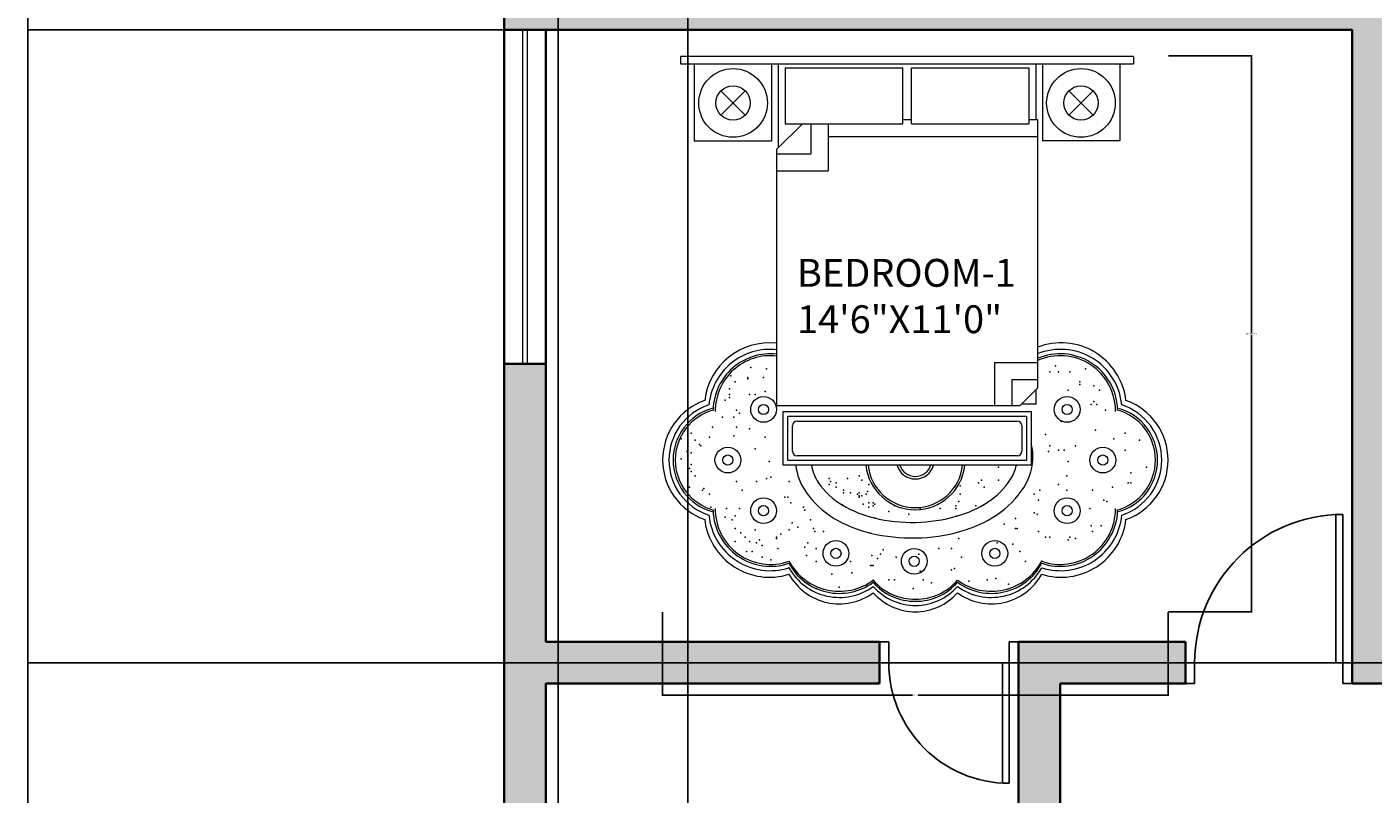
# Model space of a CAD drawing. Units: inches. Extents: x 5716 to 6907, y 12769 to 13594.
# Tile 6 of 17: x 5716 to 6007, y 13266 to 13432. Entities that reach past the tile are written whole.
import ezdxf

# ---------------------------------------------------------------- set-up
doc = ezdxf.new("R2010")
doc.units = ezdxf.units.IN
for name, color, linetype, lineweight in [('A-ANNO-DIMS', 2, 'Continuous', 18), ('A-AREA-IDEN', 7, 'Continuous', 18), ('A-DOOR', 4, 'Continuous', 25), ('A-FURN', 8, 'Continuous', 18), ('A-GLAZ', 4, 'Continuous', 18), ('A-WALL', 7, 'Continuous', 35), ('A-WALL-PATT', 252, 'Continuous', 13)]:
    doc.layers.add(name, color=color, linetype=linetype, lineweight=lineweight)
doc.styles.get("Standard").update_dxf_attribs({"font": 'arial.ttf'})
doc.dimstyles.get("Standard").update_dxf_attribs({"dimtxt": 0.18, "dimasz": 0.18, "dimexe": 0.18, "dimexo": 0.0625, "dimgap": 0.09, "dimtad": 0, "dimtih": 1, "dimtoh": 1, "dimdec": 4, "dimzin": 0, "dimdsep": 46, "dimtxsty": 'Standard', "dimcen": 0.09, "dimadec": 0, "dimazin": 0, "dimtfac": 1, "dimtdec": 4, "dimtofl": 0, "dimtmove": 0, "dimatfit": 3, "dimfxl": 1, "dimtolj": 1, "dimtzin": 0, "dimarcsym": 0})

# ---------------------------------------------------------------- blocks, each defined once
blk = doc.blocks.new('A$C1EC128A1')
for p, q in [((0.1147, 3.56), (3.0187, 3.56)), ((0.1147, 3.555), (0.1147, 3.511)), ((3.0187, 3.555), (3.0187, 3.511)), ((0.1147, 3.511), (3.0187, 3.511)), ((0.2027, 3.511), (0.2027, 3.4616)), ((0.2027, 3.4601), (0.2027, 3.016)), ((0.6977, 3.511), (0.6977, 3.016)), ((0.7417, 3.511), (0.7417, 2.972)), ((0.7857, 3.4835), (1.5392, 3.4835)), ((0.7857, 3.4835), (0.7857, 3.126)), ((1.5392, 3.126), (1.5392, 3.4835)), ((1.5942, 3.126), (1.5942, 3.4835)), ((1.5942, 3.4835), (2.3477, 3.4835)), ((2.3477, 3.4835), (2.3477, 3.126)), ((2.3917, 3.511), (2.3917, 3.1535)), ((2.4357, 3.511), (2.4357, 3.016)), ((2.9307, 3.511), (2.9307, 3.016)), ((0.3741, 3.1815), (0.5297, 3.337)), ((0.3741, 3.337), (0.5297, 3.1815)), ((2.6038, 3.337), (2.7594, 3.1815)), ((2.7594, 3.337), (2.6038, 3.1815)), ((0.7307, 2.961), (0.8957, 3.126)), ((0.7857, 3.126), (1.5392, 3.126)), ((0.9507, 3.126), (0.9507, 2.9335)), ((1.0607, 3.126), (1.0607, 2.8235)), ((1.5392, 3.1535), (1.5942, 3.1535)), ((1.5942, 3.126), (2.3477, 3.126)), ((2.3477, 3.1535), (2.4027, 3.1535)), ((2.4027, 3.1535), (2.4027, 1.432)), ((1.0607, 3.0435), (2.4027, 3.0435)), ((0.2027, 3.016), (0.6977, 3.016)), ((0.7307, 2.961), (0.7307, 1.322)), ((2.9307, 3.016), (2.4357, 3.016)), ((0.7307, 2.9335), (0.9507, 2.9335)), ((0.7307, 2.8235), (1.0607, 2.8235)), ((2.1277, 1.597), (2.4027, 1.597)), ((2.1277, 1.597), (2.1277, 1.322)), ((2.2377, 1.487), (2.2377, 1.322)), ((2.2377, 1.487), (2.4027, 1.487)), ((2.2927, 1.322), (2.4027, 1.432)), ((2.3917, 1.421), (2.3917, 1.333)), ((0.7307, 1.322), (2.2927, 1.322)), ((2.3037, 1.333), (2.3917, 1.333)), ((0.7721, 1.282), (2.3633, 1.282)), ((0.7721, 0.939), (0.7721, 1.282)), ((0.8021, 1.252), (2.3333, 1.252)), ((0.8021, 0.969), (0.8021, 1.252)), ((0.8621, 1.222), (2.2733, 1.222)), ((2.3333, 1.252), (2.3333, 0.969)), ((2.3633, 1.282), (2.3633, 0.939)), ((0.8321, 1.029), (0.8321, 1.192)), ((2.3033, 1.192), (2.3033, 1.029)), ((2.3333, 0.969), (0.8021, 0.969)), ((2.2733, 0.999), (0.8621, 0.999)), ((2.3633, 0.939), (0.7721, 0.939))]:
    blk.add_line(p, q)
for centre, radius in [((0.4519, 3.2593), 0.22), ((2.6816, 3.2593), 0.22), ((0.4519, 3.2593), 0.11), ((2.6816, 3.2593), 0.11), ((0.647, 1.2961), 0.0826), ((0.647, 1.2961), 0.0326), ((2.593, 1.2961), 0.0826), ((2.593, 1.2961), 0.0326), ((0.4183, 0.9718), 0.0826), ((2.8217, 0.9718), 0.0826), ((0.4183, 0.9718), 0.0326), ((2.8217, 0.9718), 0.0326), ((0.647, 0.6475), 0.0826), ((2.593, 0.6475), 0.0826), ((0.647, 0.6475), 0.0326), ((2.593, 0.6475), 0.0326), ((1.1109, 0.3741), 0.0826), ((2.1291, 0.3741), 0.0826), ((1.1109, 0.3741), 0.0326), ((1.6128, 0.3232), 0.0826), ((1.6128, 0.3232), 0.0326), ((2.1291, 0.3741), 0.0326)]:
    blk.add_circle(centre, radius)
for centre, radius, start, end in [((0.6854, 1.3045), 0.4183, 83.78243, 173.25148), ((0.6884, 1.2877), 0.3932, 83.81567, 174.52996), ((0.6921, 1.2838), 0.369, 83.99709, 177.99757), ((0.6913, 1.2866), 0.3539, 83.60511, 180.66989), ((2.5546, 1.3045), 0.4183, 6.74852, 111.27952), ((2.5516, 1.2877), 0.3932, 5.47004, 112.24899), ((2.5479, 1.2838), 0.369, 2.00243, 113.15364), ((2.5487, 1.2866), 0.3539, 359.33011, 114.35507), ((0.4048, 0.972), 0.4048, 109.45268, 180), ((0.4119, 0.972), 0.3714, 108.02557, 180), ((0.411, 0.972), 0.3435, 105.78906, 180), ((2.829, 0.972), 0.3435, 0, 74.21094), ((2.8281, 0.972), 0.3714, 0, 71.97443), ((2.8352, 0.972), 0.4048, 0, 70.54732), ((0.4122, 0.972), 0.3312, 104.76604, 180), ((0.8621, 1.192), 0.03, 90, 180), ((2.2733, 1.192), 0.03, 0, 90), ((2.8278, 0.972), 0.3312, 0, 75.23396), ((2.0084, 0.9935), 0.365, 1.17824, 13.48124), ((0.4048, 0.972), 0.4048, 180, 250.54732), ((0.4119, 0.972), 0.3714, 180, 251.97443), ((0.411, 0.972), 0.3435, 180, 254.21094), ((0.4122, 0.972), 0.3312, 180, 255.23396), ((0.8621, 1.029), 0.03, 180, 270), ((2.2733, 1.029), 0.03, 270, 0), ((2.0084, 0.9935), 0.365, 327.62391, 1.17824), ((2.8278, 0.972), 0.3312, 284.76604, 0), ((2.829, 0.972), 0.3435, 285.78906, 0), ((2.8281, 0.972), 0.3714, 288.02557, 0), ((2.8352, 0.972), 0.4048, 289.45268, 0), ((1.2169, 0.9773), 0.365, 186.01972, 214.73257), ((1.2169, 0.9773), 0.265, 188.30546, 214.73257), ((1.62, 0.972), 0.3185, 185.95071, 354.04929), ((1.62, 0.972), 0.305, 186.21512, 353.78488), ((1.62, 0.972), 0.1215, 195.7695, 344.2305), ((1.62, 0.972), 0.105, 198.32909, 341.67091), ((2.0084, 0.9935), 0.265, 327.62391, 348.11864), ((1.4035, 1.1066), 0.492, 214.73257, 239.1926), ((1.8167, 1.1151), 0.492, 303.16388, 327.62391), ((1.8167, 1.1151), 0.592, 303.16388, 327.62391), ((1.4035, 1.1066), 0.592, 214.73257, 239.1926), ((1.6878, 1.3123), 0.7275, 285.68186, 303.16388), ((0.6884, 0.6563), 0.3932, 185.47004, 288.01752), ((0.6921, 0.6602), 0.369, 182.00243, 288.62304), ((0.6913, 0.6574), 0.3539, 179.33011, 289.59453), ((1.5241, 1.3089), 0.7275, 239.1926, 256.67462), ((1.5995, 1.627), 1.0544, 271.17824, 285.68186), ((1.6878, 1.3123), 0.8275, 285.68186, 303.16388), ((2.5487, 0.6574), 0.3539, 250.40547, 0.66989), ((2.5479, 0.6602), 0.369, 251.37696, 357.99757), ((2.5516, 0.6563), 0.3932, 251.98248, 354.52996), ((0.6854, 0.6395), 0.4183, 186.74852, 287.32326), ((1.5241, 1.3089), 0.8275, 239.1926, 256.67462), ((1.5995, 1.627), 1.0544, 256.67462, 271.17824), ((2.5546, 0.6395), 0.4183, 252.67674, 353.25148), ((1.5995, 1.627), 1.1544, 256.67462, 271.17824), ((1.5995, 1.627), 1.1544, 271.17824, 285.68186), ((1.1328, 0.4977), 0.3665, 208.29135, 306.34788), ((1.1328, 0.4842), 0.3665, 208.29135, 306.34788), ((1.133, 0.4609), 0.369, 208.93019, 306.02618), ((2.1072, 0.4977), 0.3665, 233.65212, 331.70865), ((2.1072, 0.4842), 0.3665, 233.65212, 331.70865), ((2.107, 0.4609), 0.369, 233.97382, 331.06981), ((1.1324, 0.4204), 0.3694, 209.22014, 306.07902), ((1.6145, 0.4295), 0.3486, 220.6393, 270.90521), ((1.6145, 0.416), 0.3486, 220.6393, 270.90521), ((1.6255, 0.4295), 0.3486, 269.09479, 319.3607), ((1.6255, 0.416), 0.3486, 269.09479, 319.3607), ((2.1076, 0.4204), 0.3694, 233.92098, 330.77986), ((1.62, 0.4004), 0.3599, 221.38778, 270), ((1.62, 0.36), 0.36, 221.41854, 270), ((1.62, 0.4004), 0.3599, 270, 318.61222), ((1.62, 0.36), 0.36, 270, 318.58146)]:
    blk.add_arc(centre, radius, start, end)
for p in [(0.5654, 1.5652), (0.6657, 1.5561), (2.5184, 1.5744), (2.71, 1.5561), (0.4376, 1.5104), (0.465, 1.4739), (0.5471, 1.5013), (0.5471, 1.4922), (0.6475, 1.5013), (2.4819, 1.5378), (2.5366, 1.5378), (2.6097, 1.5378), (2.6735, 1.4739), (0.4285, 1.4282), (0.4285, 1.3917), (0.5562, 1.3917), (0.5927, 1.3917), (0.6566, 1.41), (2.6005, 1.4191), (2.6735, 1.4556), (2.7648, 1.4465), (2.8013, 1.4191), (0.4011, 1.3552), (0.4285, 1.3734), (2.3917, 1.333), (2.7465, 1.3278), (2.7648, 1.346), (2.7831, 1.3278), (0.3828, 1.2456), (0.4558, 1.2456), (0.4741, 1.2912), (0.4923, 1.273), (2.5549, 1.2182), (2.8378, 1.2912), (0.1821, 1.1451), (0.3189, 1.1816), (0.4558, 1.1268), (0.4741, 1.1816), (0.5562, 1.1725), (2.4545, 1.1359), (2.7739, 1.1634), (2.9656, 1.1451), (0.1182, 1.1085), (0.2094, 1.0994), (0.2368, 1.072), (0.2459, 1.0629), (0.3007, 1.1177), (0.5927, 1.0446), (0.6566, 1.1177), (2.4819, 1.0629), (2.5366, 1.0355), (2.5731, 1.0355), (2.6462, 1.0629), (2.8926, 1.1085), (2.9656, 1.0355), (3.0568, 1.0994), (0.1182, 0.9807), (0.1547, 1.0263), (0.1821, 1.0172), (0.684, 0.9624), (2.4728, 1.0263), (2.6005, 0.9624), (0.1729, 0.9167), (0.1821, 0.9441), (0.1821, 0.8985), (0.2094, 0.8711), (1.259, 0.8711), (1.3032, 0.939), (1.3168, 0.939), (2.1533, 0.9259), (2.5914, 0.8711), (3.0021, 0.8893), (3.1025, 0.9259), (0.1729, 0.798), (0.2551, 0.7797), (0.2642, 0.7889), (0.4741, 0.8345), (0.5106, 0.7797), (0.6019, 0.8345), (0.6657, 0.8528), (0.6931, 0.8619), (0.8118, 0.8345), (0.9992, 0.8263), (1.0673, 0.8528), (1.0673, 0.8163), (1.0764, 0.8345), (1.1129, 0.8254), (1.1129, 0.798), (1.1586, 0.7797), (1.1859, 0.8528), (1.2772, 0.8437), (1.3228, 0.8163), (1.9069, 0.8071), (2.0256, 0.8254), (2.0438, 0.8437), (2.0438, 0.8437), (2.0621, 0.798), (2.1533, 0.8437), (2.418, 0.7797), (2.5366, 0.8163), (2.5914, 0.7797), (2.7557, 0.7797), (2.8834, 0.798), (2.9838, 0.8254), (3.0021, 0.8254), (0.3007, 0.7523), (0.7844, 0.7341), (0.8026, 0.7341), (0.8209, 0.6975), (1.1586, 0.7615), (1.2042, 0.7615), (1.2498, 0.7523), (1.259, 0.7615), (1.259, 0.7432), (1.259, 0.7341), (1.2772, 0.7432), (1.3046, 0.7523), (1.3137, 0.7706), (1.3228, 0.6975), (1.3502, 0.6975), (1.8978, 0.7067), (1.9069, 0.7523), (2.0858, 0.7033), (2.3815, 0.7523), (2.4089, 0.7158), (2.8287, 0.7158), (2.8469, 0.7067), (0.3098, 0.6701), (0.4011, 0.6062), (0.4102, 0.661), (0.465, 0.6153), (0.4923, 0.661), (0.903, 0.6701), (0.9122, 0.6519), (1.1515, 0.684), (1.1515, 0.684), (1.1515, 0.684), (1.2863, 0.6884), (1.3228, 0.6701), (1.3502, 0.6793), (1.3593, 0.6884), (1.4506, 0.6427), (1.4871, 0.6793), (1.5784, 0.6245), (1.6514, 0.661), (1.6514, 0.661), (1.7792, 0.661), (1.8795, 0.6793), (1.8795, 0.661), (1.8845, 0.6118), (2.0073, 0.6793), (2.3815, 0.6336), (2.3997, 0.6245), (2.7374, 0.661), (0.4467, 0.5879), (0.465, 0.5331), (0.5927, 0.524), (0.8118, 0.524), (0.83, 0.5696), (0.8665, 0.5422), (0.9487, 0.5879), (0.9669, 0.5331), (1.3564, 0.601), (2.1898, 0.5605), (2.2629, 0.597), (2.2629, 0.5331), (2.272, 0.5331), (2.7465, 0.5514), (2.8104, 0.5514), (0.465, 0.4509), (0.5015, 0.5057), (0.5289, 0.4783), (0.5562, 0.4509), (0.6019, 0.4418), (0.6201, 0.46), (0.7296, 0.4783), (0.7296, 0.4692), (0.757, 0.4966), (0.9304, 0.4418), (0.976, 0.5148), (1.0308, 0.5148), (1.3334, 0.5037), (1.8978, 0.4692), (2.1442, 0.4418), (2.2446, 0.4326), (2.4089, 0.5148), (2.4545, 0.4783), (2.4819, 0.4783), (2.6005, 0.46), (2.6097, 0.4783), (2.6462, 0.4692), (2.7557, 0.5148), (0.538, 0.387), (0.5745, 0.387), (0.6384, 0.4235), (0.6384, 0.3504), (0.7388, 0.4052), (0.7388, 0.4052), (0.9122, 0.4144), (0.9213, 0.3596), (0.9852, 0.4052), (1.3411, 0.3596), (1.3959, 0.3687), (1.4141, 0.3961), (1.4962, 0.3504), (1.6423, 0.3687), (1.77, 0.4052), (1.8522, 0.4052), (1.9161, 0.3504), (2.2902, 0.387), (0.6931, 0.3322), (0.81, 0.2824), (0.9852, 0.323), (1.2042, 0.323), (1.332, 0.2956), (1.3411, 0.2956), (1.3502, 0.2956), (1.3776, 0.3413), (1.6514, 0.2591), (1.8522, 0.2682), (1.8704, 0.2774), (2.3267, 0.323), (2.43, 0.324), (1.0856, 0.2408), (1.2133, 0.25), (1.35, 0.2025), (1.4506, 0.2043), (1.4871, 0.2043), (1.6696, 0.2043), (1.7244, 0.186), (1.9617, 0.1952), (2.0803, 0.2043), (2.1351, 0.2134), (2.2172, 0.1769), (0.9852, 0.1495), (1.1312, 0.1586), (1.6058, 0.1495)]:
    blk.add_point(p)
blk = doc.blocks.new('DOOR-SWING-30IN')
for p, q in [((0, 4.5), (-2, 4.5)), ((0, 0), (0, 4.5)), ((26, 0), (26, 4.5)), ((26, 4.5), (28, 4.5)), ((-2, 0), (0, 0)), ((0, -26), (0, 0)), ((0, 0), (1.5, 0)), ((1.5, -25.96), (1.5, 0)), ((28, 0), (26, 0))]:
    blk.add_line(p, q)
blk.add_arc((0, 0), 26, 270, 0)
blk = doc.blocks.new('DOOR-SWING-36IN')
for p, q in [((0, 32), (0, 0)), ((1.5, 31.96), (1.5, 0)), ((-2, 0), (0, 0)), ((0, 0), (0, -4.5)), ((0, 0), (1.5, 0)), ((34, 0), (32, 0)), ((32, 0), (32, -4.5)), ((0, -4.5), (-2, -4.5)), ((32, -4.5), (34, -4.5))]:
    blk.add_line(p, q)
blk.add_arc((0, 0), 32, 0, 90)
blk = doc.blocks.new('WIN-GLAZING-72IN')
for p, q in [((0, 0), (0, -72)), ((1, 0), (1, -72))]:
    blk.add_line(p, q)
blk = doc.blocks.new('*D27')
at = {"layer": 'A-ANNO-DIMS', "color": 0, "lineweight": -2, "transparency": 16777216}
for p, q in [((5962.35, 13425.52), (5980.45, 13425.52)), ((5980.27, 13425.34), (5980.27, 13365.77)), ((5980.27, 13305.83), (5980.27, 13365.4)), ((5962.35, 13305.65), (5980.45, 13305.65))]:
    blk.add_line(p, q, dxfattribs=at)
at = {"layer": 'A-ANNO-DIMS', "color": 0, "transparency": 16777216}
for points in [[(5980.24, 13425.34), (5980.3, 13425.34), (5980.27, 13425.52)], [(5980.24, 13305.83), (5980.3, 13305.83), (5980.27, 13305.65)]]:
    blk.add_solid(points, dxfattribs=at)
at = {"layer": 'Defpoints', "color": 0, "transparency": 16777216}
for p in [(5962.29, 13425.52), (5980.27, 13425.52), (5962.29, 13305.65)]:
    blk.add_point(p, dxfattribs=at)
at = {"layer": 'A-ANNO-DIMS', "color": 0, "transparency": 16777216, "insert": (5980.27, 13365.59), "char_height": 0.18, "attachment_point": 5}
blk.add_mtext('\\A1;BED GROUP 120 TYP.', dxfattribs=at)
blk = doc.blocks.new('*D28')
at = {"layer": 'A-ANNO-DIMS', "color": 0, "lineweight": -2, "transparency": 16777216}
for p, q in [((5853.2, 13305.59), (5853.2, 13287.49)), ((5962.29, 13305.59), (5962.29, 13287.49)), ((5853.38, 13287.67), (5907.16, 13287.67)), ((5962.11, 13287.67), (5908.34, 13287.67))]:
    blk.add_line(p, q, dxfattribs=at)
at = {"layer": 'A-ANNO-DIMS', "color": 0, "transparency": 16777216}
for points in [[(5853.38, 13287.7), (5853.38, 13287.64), (5853.2, 13287.67)], [(5962.11, 13287.7), (5962.11, 13287.64), (5962.29, 13287.67)]]:
    blk.add_solid(points, dxfattribs=at)
at = {"layer": 'Defpoints', "color": 0, "transparency": 16777216}
for p in [(5853.2, 13305.65), (5962.29, 13305.65), (5962.29, 13287.67)]:
    blk.add_point(p, dxfattribs=at)
at = {"layer": 'A-ANNO-DIMS', "color": 0, "transparency": 16777216, "insert": (5907.75, 13287.67), "char_height": 0.18, "attachment_point": 5}
blk.add_mtext('\\A1;109 TYP.', dxfattribs=at)
blk = doc.blocks.new('*D50')
at = {"layer": 'A-ANNO-DIMS', "color": 0, "lineweight": -2, "transparency": 16777216}
for p, q in [((5818.96, 13440.15), (5716.04, 13440.15)), ((5716.22, 13439.97), (5716.22, 13140.83)), ((5716.22, 12841.33), (5716.22, 13140.47)), ((5818.96, 12841.15), (5716.04, 12841.15))]:
    blk.add_line(p, q, dxfattribs=at)
at = {"layer": 'A-ANNO-DIMS', "color": 0, "transparency": 16777216}
for points in [[(5716.19, 13439.97), (5716.25, 13439.97), (5716.22, 13440.15)], [(5716.19, 12841.33), (5716.25, 12841.33), (5716.22, 12841.15)]]:
    blk.add_solid(points, dxfattribs=at)
at = {"layer": 'Defpoints', "color": 0, "transparency": 16777216}
for p in [(5716.22, 13440.15), (5819.02, 13440.15), (5819.02, 12841.15)]:
    blk.add_point(p, dxfattribs=at)
at = {"layer": 'A-ANNO-DIMS', "color": 0, "transparency": 16777216, "insert": (5716.22, 13140.65), "char_height": 0.18, "attachment_point": 5}
blk.add_mtext('\\A1;599', dxfattribs=at)
blk = doc.blocks.new('*D51')
at = {"layer": 'A-ANNO-DIMS', "color": 0, "lineweight": -2, "transparency": 16777216}
for p, q in [((5819.02, 13440.21), (5819.02, 13594.38)), ((5819.2, 13594.2), (6033.23, 13594.2)), ((6247.84, 13594.2), (6033.82, 13594.2)), ((6248.02, 13194.21), (6248.02, 13594.38))]:
    blk.add_line(p, q, dxfattribs=at)
at = {"layer": 'A-ANNO-DIMS', "color": 0, "transparency": 16777216}
for points in [[(5819.2, 13594.23), (5819.2, 13594.17), (5819.02, 13594.2)], [(6247.84, 13594.23), (6247.84, 13594.17), (6248.02, 13594.2)]]:
    blk.add_solid(points, dxfattribs=at)
at = {"layer": 'Defpoints', "color": 0, "transparency": 16777216}
for p in [(6248.02, 13594.2), (5819.02, 13440.15), (6248.02, 13194.15)]:
    blk.add_point(p, dxfattribs=at)
at = {"layer": 'A-ANNO-DIMS', "color": 0, "transparency": 16777216, "insert": (6033.52, 13594.2), "char_height": 0.18, "attachment_point": 5}
blk.add_mtext('\\A1;429', dxfattribs=at)
blk = doc.blocks.new('*D52')
at = {"layer": 'A-ANNO-DIMS', "color": 0, "lineweight": -2, "transparency": 16777216}
for p, q in [((6267.34, 13440.15), (5716.04, 13440.15)), ((5716.22, 13439.97), (5716.22, 13140.83)), ((5716.22, 12841.33), (5716.22, 13140.47)), ((6267.34, 12841.15), (5716.04, 12841.15))]:
    blk.add_line(p, q, dxfattribs=at)
at = {"layer": 'A-ANNO-DIMS', "color": 0, "transparency": 16777216}
for points in [[(5716.19, 13439.97), (5716.25, 13439.97), (5716.22, 13440.15)], [(5716.19, 12841.33), (5716.25, 12841.33), (5716.22, 12841.15)]]:
    blk.add_solid(points, dxfattribs=at)
at = {"layer": 'Defpoints', "color": 0, "transparency": 16777216}
for p in [(6267.41, 13440.15), (5716.22, 12841.15), (6267.41, 12841.15)]:
    blk.add_point(p, dxfattribs=at)
at = {"layer": 'A-ANNO-DIMS', "color": 0, "transparency": 16777216, "insert": (5716.22, 13140.65), "char_height": 0.18, "attachment_point": 5}
blk.add_mtext('\\A1;599', dxfattribs=at)
blk = doc.blocks.new('*D58')
at = {"layer": 'A-ANNO-DIMS', "color": 0, "lineweight": -2, "transparency": 16777216}
for p, q in [((6736.67, 13435.65), (5716.04, 13435.65)), ((5716.22, 13435.47), (5716.22, 13365.33)), ((5716.22, 13294.83), (5716.22, 13364.97)), ((6736.67, 13294.65), (5716.04, 13294.65))]:
    blk.add_line(p, q, dxfattribs=at)
at = {"layer": 'A-ANNO-DIMS', "color": 0, "transparency": 16777216}
for points in [[(5716.19, 13435.47), (5716.25, 13435.47), (5716.22, 13435.65)], [(5716.19, 13294.83), (5716.25, 13294.83), (5716.22, 13294.65)]]:
    blk.add_solid(points, dxfattribs=at)
at = {"layer": 'Defpoints', "color": 0, "transparency": 16777216}
for p in [(6736.73, 13435.65), (5716.22, 13294.65), (6736.73, 13294.65)]:
    blk.add_point(p, dxfattribs=at)
at = {"layer": 'A-ANNO-DIMS', "color": 0, "transparency": 16777216, "insert": (5716.22, 13365.15), "char_height": 0.18, "attachment_point": 5}
blk.add_mtext('\\A1;141', dxfattribs=at)
blk = doc.blocks.new('*D59')
at = {"layer": 'A-ANNO-DIMS', "color": 0, "lineweight": -2, "transparency": 16777216}
for p, q in [((6736.67, 13294.65), (5716.04, 13294.65)), ((5716.22, 13294.47), (5716.22, 13248.33)), ((5716.22, 13201.83), (5716.22, 13247.97)), ((6736.67, 13201.65), (5716.04, 13201.65))]:
    blk.add_line(p, q, dxfattribs=at)
at = {"layer": 'A-ANNO-DIMS', "color": 0, "transparency": 16777216}
for points in [[(5716.19, 13294.47), (5716.25, 13294.47), (5716.22, 13294.65)], [(5716.19, 13201.83), (5716.25, 13201.83), (5716.22, 13201.65)]]:
    blk.add_solid(points, dxfattribs=at)
at = {"layer": 'Defpoints', "color": 0, "transparency": 16777216}
for p in [(6736.73, 13294.65), (5716.22, 13201.65), (6736.73, 13201.65)]:
    blk.add_point(p, dxfattribs=at)
at = {"layer": 'A-ANNO-DIMS', "color": 0, "transparency": 16777216, "insert": (5716.22, 13248.15), "char_height": 0.18, "attachment_point": 5}
blk.add_mtext('\\A1;93', dxfattribs=at)
blk = doc.blocks.new('*D65')
at = {"layer": 'A-ANNO-DIMS', "color": 0, "lineweight": -2, "transparency": 16777216}
for p, q in [((5818.96, 13440.15), (5716.04, 13440.15)), ((5716.22, 13439.97), (5716.22, 13435.83)), ((5716.22, 13431.33), (5716.22, 13435.47)), ((5827.96, 13431.15), (5716.04, 13431.15))]:
    blk.add_line(p, q, dxfattribs=at)
at = {"layer": 'A-ANNO-DIMS', "color": 0, "transparency": 16777216}
for points in [[(5716.19, 13439.97), (5716.25, 13439.97), (5716.22, 13440.15)], [(5716.19, 13431.33), (5716.25, 13431.33), (5716.22, 13431.15)]]:
    blk.add_solid(points, dxfattribs=at)
at = {"layer": 'Defpoints', "color": 0, "transparency": 16777216}
for p in [(5819.02, 13440.15), (5716.22, 13431.15), (5828.02, 13431.15)]:
    blk.add_point(p, dxfattribs=at)
at = {"layer": 'A-ANNO-DIMS', "color": 0, "transparency": 16777216, "insert": (5716.22, 13435.65), "char_height": 0.18, "attachment_point": 5}
blk.add_mtext('\\A1;9', dxfattribs=at)
blk = doc.blocks.new('*D75')
at = {"layer": 'A-ANNO-DIMS', "color": 0, "lineweight": -2, "transparency": 16777216}
for p, q in [((5830.67, 13257.62), (5830.67, 13594.38)), ((5830.85, 13594.2), (5844.45, 13594.2)), ((5858.49, 13594.2), (5844.89, 13594.2)), ((5858.67, 13247.12), (5858.67, 13594.38))]:
    blk.add_line(p, q, dxfattribs=at)
at = {"layer": 'A-ANNO-DIMS', "color": 0, "transparency": 16777216}
for points in [[(5830.85, 13594.23), (5830.85, 13594.17), (5830.67, 13594.2)], [(5858.49, 13594.23), (5858.49, 13594.17), (5858.67, 13594.2)]]:
    blk.add_solid(points, dxfattribs=at)
at = {"layer": 'Defpoints', "color": 0, "transparency": 16777216}
for p in [(5858.67, 13594.2), (5830.67, 13257.56), (5858.67, 13247.06)]:
    blk.add_point(p, dxfattribs=at)
at = {"layer": 'A-ANNO-DIMS', "color": 0, "transparency": 16777216, "insert": (5844.67, 13594.2), "char_height": 0.18, "attachment_point": 5}
blk.add_mtext('\\A1;28', dxfattribs=at)

msp = doc.modelspace()

# ---------------------------------------------------------------- hatches: boundary and pattern name
at = {"layer": 'A-WALL-PATT'}
h = msp.add_hatch(color=256, dxfattribs=at)
h.dxf.hatch_style = 1
h.paths.add_polyline_path([(6188.02, 13440.15), (5819.02, 13440.15), (5819.02, 13431.15), (6002.02, 13431.15), (6002.02, 13290.15), (6011.02, 13290.15), (6011.02, 13431.15), (6188.02, 13431.15)])
h = msp.add_hatch(color=256, dxfattribs=at)
h.dxf.hatch_style = 1
h.paths.add_polyline_path([(5828.02, 13359.15), (5819.02, 13359.15), (5819.02, 13260.15), (5828.02, 13260.15), (5828.02, 13290.15), (5900.02, 13290.15), (5900.02, 13299.15), (5828.02, 13299.15)])
h = msp.add_hatch(color=256, dxfattribs=at)
h.dxf.hatch_style = 1
h.paths.add_polyline_path([(5939.02, 13290.15), (5966.02, 13290.15), (5966.02, 13299.15), (5930.02, 13299.15), (5930.02, 13206.15), (5828.02, 13206.15), (5828.02, 13236.15), (5819.02, 13236.15), (5819.02, 13173.15), (5828.02, 13173.15), (5828.02, 13197.15), (5930.02, 13197.15), (5930.02, 13116.15), (5939.02, 13116.15)])

# ---------------------------------------------------------------- linework, layer by layer
at = {"layer": 'A-WALL'}
for p, q in [((5819.02, 13440.15), (5819.02, 12841.15)), ((5819.02, 13431.15), (6002.02, 13431.15)), ((5828.02, 13431.15), (5828.02, 13299.15)), ((6002.02, 13431.15), (6002.02, 13290.15)), ((5819.02, 13359.15), (5828.02, 13359.15)), ((5828.02, 13299.15), (5900.02, 13299.15)), ((5900.02, 13299.15), (5900.02, 13290.15)), ((5930.02, 13299.15), (5930.02, 13206.15)), ((5930.02, 13299.15), (5966.02, 13299.15)), ((5966.02, 13299.15), (5966.02, 13290.15)), ((5828.02, 13290.15), (5900.02, 13290.15)), ((5828.02, 13290.15), (5828.02, 13206.15)), ((5939.02, 13290.15), (5939.02, 13116.15)), ((5939.02, 13290.15), (5966.02, 13290.15)), ((6002.02, 13290.15), (6011.02, 13290.15))]:
    msp.add_line(p, q, dxfattribs=at)

# ---------------------------------------------------------------- block references
at = {"layer": 'A-DOOR', "extrusion": (0, 0, -1), "zscale": -1}
for name, p in [('DOOR-SWING-36IN', (-6000.02, 13294.65)), ('DOOR-SWING-30IN', (-5928.02, 13294.65))]:
    msp.add_blockref(name, p, dxfattribs=at)
at = {"layer": 'A-FURN', "xscale": 33.66910864864256, "yscale": 33.66910864864256, "zscale": 33.66910864864256}
msp.add_blockref('A$C1EC128A1', (5853.2, 13305.65), dxfattribs=at)
at = {"layer": 'A-GLAZ', "rotation": 180}
msp.add_blockref('WIN-GLAZING-72IN', (5824.02, 13359.15), dxfattribs=at)

# ---------------------------------------------------------------- texts
at = {"layer": 'A-AREA-IDEN', "insert": (5882.2, 13381.75), "char_height": 6, "attachment_point": 1}
msp.add_mtext_dynamic_manual_height_columns('BEDROOM-1\\P14\'6"X11\'0"', width=112.0121, gutter_width=12.5, heights=[0], dxfattribs=at)

# ---------------------------------------------------------------- dimensions: what is measured, and where the dimension line sits
at = {"layer": 'A-ANNO-DIMS'}
for base, p1, p2, picture, middle in [((6248.02, 13594.2), (5819.02, 13440.15), (6248.02, 13194.15), '*D51', (6033.52, 13594.2)), ((5858.67, 13594.2), (5830.67, 13257.56), (5858.67, 13247.06), '*D75', (5844.67, 13594.2))]:
    dim = msp.add_linear_dim(base=base, p1=p1, p2=p2, dimstyle='Standard', override={"dimdec": 0, "dimlfac": 1, "dimrnd": 0, "dimzin": 0, "dimdsep": 46, "dimlunit": 2}, dxfattribs=at)
    dim.commit()
    dim.dimension.update_dxf_attribs({"geometry": picture, "text_midpoint": middle})
for base, p1, p2, picture, middle in [((5716.22, 13440.15), (5819.02, 12841.15), (5819.02, 13440.15), '*D50', (5716.22, 13140.65)), ((5716.22, 12841.15), (6267.41, 13440.15), (6267.41, 12841.15), '*D52', (5716.22, 13140.65)), ((5716.22, 13431.15), (5819.02, 13440.15), (5828.02, 13431.15), '*D65', (5716.22, 13435.65)), ((5716.22, 13294.65), (6736.73, 13435.65), (6736.73, 13294.65), '*D58', (5716.22, 13365.15)), ((5716.22, 13201.65), (6736.73, 13294.65), (6736.73, 13201.65), '*D59', (5716.22, 13248.15))]:
    dim = msp.add_linear_dim(base=base, p1=p1, p2=p2, angle=90, dimstyle='Standard', override={"dimdec": 0, "dimlfac": 1, "dimrnd": 0, "dimzin": 0, "dimdsep": 46, "dimlunit": 2}, dxfattribs=at)
    dim.commit()
    dim.dimension.update_dxf_attribs({"geometry": picture, "text_midpoint": middle})
dim = msp.add_linear_dim(base=(5980.27, 13425.52), p1=(5962.29, 13305.65), p2=(5962.29, 13425.52), angle=90, text='BED GROUP <> TYP.', dimstyle='Standard', override={"dimdec": 0, "dimlfac": 1, "dimrnd": 0, "dimzin": 0, "dimdsep": 46, "dimlunit": 2}, dxfattribs=at)
dim.commit()
dim.dimension.update_dxf_attribs({"geometry": '*D27', "text_midpoint": (5980.27, 13365.59)})
dim = msp.add_linear_dim(base=(5962.29, 13287.67), p1=(5853.2, 13305.65), p2=(5962.29, 13305.65), text='<> TYP.', dimstyle='Standard', override={"dimdec": 0, "dimlfac": 1, "dimrnd": 0, "dimzin": 0, "dimdsep": 46, "dimlunit": 2}, dxfattribs=at)
dim.commit()
dim.dimension.update_dxf_attribs({"geometry": '*D28', "text_midpoint": (5907.75, 13287.67)})

doc.saveas('drawing.dxf')
